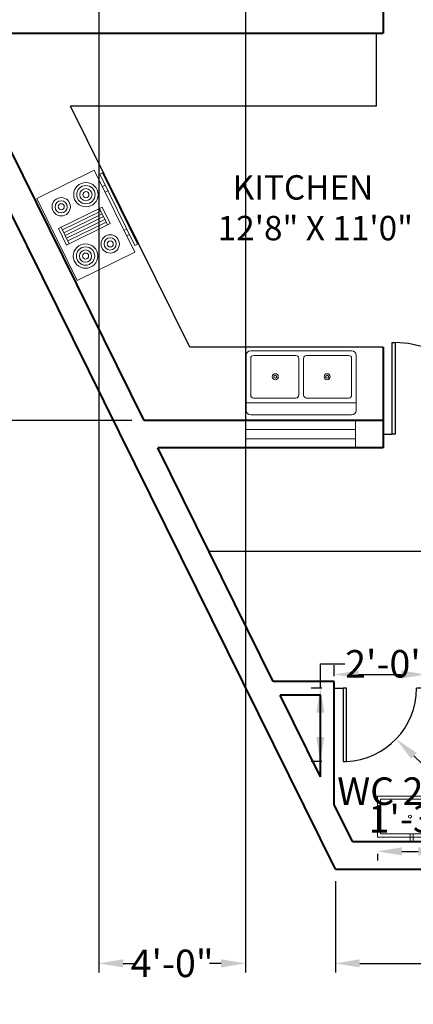
# Model space of a CAD drawing. Units: inches. Extents: x 927 to 1540, y 259 to 890.
# Tile 2 of 4: x 1137 to 1265, y 259 to 582. Entities that reach past the tile are written whole.
import ezdxf

# ---------------------------------------------------------------- set-up
doc = ezdxf.new("R2010")
doc.units = ezdxf.units.IN
doc.header["$MEASUREMENT"] = 0
for name, color, linetype, lineweight in [('A-ANNO-DIMS', 2, 'Continuous', 18), ('A-AREA-IDEN', 7, 'Continuous', 25), ('A-DOOR', 3, 'Continuous', 25), ('A-EQPM', 8, 'Continuous', 18), ('A-EQPM-PATT', 8, 'Continuous', 13), ('A-FLOR-CASE', 9, 'Continuous', 25), ('A-FLOR-FIXT', 9, 'Continuous', 18), ('A-FLOR-STRS', 7, 'Continuous', 25), ('A-GLAZ', 4, 'Continuous', 18), ('A-WALL', 7, 'Continuous', 40)]:
    doc.layers.add(name, color=color, linetype=linetype, lineweight=lineweight)
doc.styles.get("Standard").update_dxf_attribs({"font": 'arial.ttf'})
doc.dimstyles.get("Standard").update_dxf_attribs({"dimtxt": 9, "dimasz": 8, "dimexe": 3, "dimexo": 4, "dimgap": 0.09, "dimtad": 0, "dimtih": 1, "dimtoh": 1, "dimdec": 0, "dimzin": 0, "dimdsep": 46, "dimlunit": 3, "dimtxsty": 'Standard', "dimcen": 0.09, "dimadec": 0, "dimazin": 0, "dimtfac": 1, "dimtdec": 0, "dimtofl": 0, "dimtmove": 0, "dimatfit": 3, "dimfxl": 1, "dimtolj": 1, "dimtzin": 0, "dimarcsym": 0})

# ---------------------------------------------------------------- blocks, each defined once
blk = doc.blocks.new('DOOR-SINGLE-36-OPENING')
for p, q in [((3, 0), (3, 30)), ((3, 30), (4, 30)), ((4, 30), (4, 0)), ((0, 0), (3, 0)), ((4, 0), (3, 0)), ((36, 0), (33, 0))]:
    blk.add_line(p, q)
blk.add_arc((4, 0.98), 29.02, 358.058, 90)
blk = doc.blocks.new('DOOR-SINGLE-30-OPENING')
for p, q in [((0, 24), (3, 24)), ((3, 24), (3, 0)), ((4, 24), (3, 24)), ((4, 0), (4, 24)), ((30, 24), (27, 24)), ((3, 0), (4, 0))]:
    blk.add_line(p, q)
blk.add_arc((2.98, 24), 24.02, 272.4378, 0)
blk = doc.blocks.new('LAVATORY-RECTANGULAR')
for p, q in [((10.69, 2.5), (10.69, 0)), ((11.69, 2.5), (11.69, 0))]:
    blk.add_line(p, q)
for points in [[(0, 1.5), (21.39, 1.5), (21.39, 14.9), (0, 14.9)], [(1, 2.5), (20.39, 2.5), (20.39, 13.9), (1, 13.9)]]:
    blk.add_lwpolyline(points, close=True)
blk.add_circle((10.69, 8.2), 0.491)
blk = doc.blocks.new('WINDOW-36')
for p, q in [((0, 9), (0, 0)), ((36, 9), (36, 0)), ((0, 6), (36, 6)), ((0, 3), (36, 3))]:
    blk.add_line(p, q)
blk = doc.blocks.new('*D34')
at = {"layer": 'A-ANNO-DIMS', "color": 0, "lineweight": -2, "transparency": 16777216}
for p, q in [((1239.48, 366.64), (1239.48, 370.14)), ((1269.48, 366.64), (1269.48, 370.14)), ((1247.48, 367.14), (1261.48, 367.14)), ((1269.48, 367.14), (1277.48, 367.14))]:
    blk.add_line(p, q, dxfattribs=at)
at = {"layer": 'A-ANNO-DIMS', "color": 0, "lineweight": 100, "transparency": 16777216}
for points in [[(1247.48, 368.47), (1247.48, 365.81), (1239.48, 367.14)], [(1261.48, 368.47), (1261.48, 365.81), (1269.48, 367.14)]]:
    blk.add_solid(points, dxfattribs=at)
at = {"layer": 'Defpoints', "color": 0, "lineweight": 100, "transparency": 16777216}
for p in [(1269.48, 367.14), (1239.48, 362.64), (1269.48, 362.64)]:
    blk.add_point(p, dxfattribs=at)
at = {"layer": 'A-ANNO-DIMS', "color": 0, "transparency": 16777216, "insert": (1349.47, 367.14), "char_height": 9, "attachment_point": 5}
blk.add_mtext('\\A1;TOILET DOOR 2\'-6" TYP.', dxfattribs=at)
blk = doc.blocks.new('*D35')
at = {"layer": 'A-ANNO-DIMS', "color": 0, "lineweight": -2, "transparency": 16777216}
for p, q in [((1234.98, 362.64), (1234.98, 370.64)), ((1234.98, 370.64), (1242.98, 370.64)), ((1235.48, 362.64), (1231.98, 362.64)), ((1234.98, 346.64), (1234.98, 354.64)), ((1235.48, 338.64), (1231.98, 338.64))]:
    blk.add_line(p, q, dxfattribs=at)
at = {"layer": 'A-ANNO-DIMS', "color": 0, "lineweight": 100, "transparency": 16777216}
for points in [[(1233.64, 354.64), (1236.31, 354.64), (1234.98, 362.64)], [(1233.64, 346.64), (1236.31, 346.64), (1234.98, 338.64)]]:
    blk.add_solid(points, dxfattribs=at)
at = {"layer": 'Defpoints', "color": 0, "lineweight": 100, "transparency": 16777216}
for p in [(1234.98, 362.64), (1239.48, 362.64), (1239.48, 338.64)]:
    blk.add_point(p, dxfattribs=at)
at = {"layer": 'A-ANNO-DIMS', "color": 0, "transparency": 16777216, "insert": (1270.57, 370.64), "char_height": 9, "attachment_point": 5}
blk.add_mtext('\\A1;2\'-0" TYP.', dxfattribs=at)
blk = doc.blocks.new('*D44')
at = {"layer": 'A-ANNO-DIMS', "color": 0, "lineweight": -2, "transparency": 16777216}
for p, q in [((1279.6, 345.44), (1275.65, 345.44)), ((1278.65, 337.44), (1278.65, 333.66)), ((1278.65, 320.39), (1278.65, 324.17)), ((1279.6, 312.39), (1275.65, 312.39))]:
    blk.add_line(p, q, dxfattribs=at)
at = {"layer": 'A-ANNO-DIMS', "color": 0, "lineweight": 100, "transparency": 16777216}
for points in [[(1277.31, 337.44), (1279.98, 337.44), (1278.65, 345.44)], [(1277.31, 320.39), (1279.98, 320.39), (1278.65, 312.39)]]:
    blk.add_solid(points, dxfattribs=at)
at = {"layer": 'Defpoints', "color": 0, "lineweight": 100, "transparency": 16777216}
for p in [(1283.6, 345.44), (1278.65, 312.39), (1283.6, 312.39)]:
    blk.add_point(p, dxfattribs=at)
at = {"layer": 'A-ANNO-DIMS', "color": 0, "transparency": 16777216, "insert": (1278.65, 328.91), "char_height": 9, "attachment_point": 5}
blk.add_mtext('\\A1;WC 2\'-9" TYP.', dxfattribs=at)
blk = doc.blocks.new('*D46')
at = {"layer": 'A-ANNO-DIMS', "color": 0, "lineweight": -2, "transparency": 16777216}
for p, q in [((1253.64, 308.39), (1253.64, 306.18)), ((1261.64, 309.18), (1267.03, 309.18)), ((1275.03, 309.18), (1283.03, 309.18)), ((1275.03, 308.39), (1275.03, 306.18))]:
    blk.add_line(p, q, dxfattribs=at)
at = {"layer": 'A-ANNO-DIMS', "color": 0, "lineweight": 100, "transparency": 16777216}
for points in [[(1261.64, 310.52), (1261.64, 307.85), (1253.64, 309.18)], [(1267.03, 310.52), (1267.03, 307.85), (1275.03, 309.18)]]:
    blk.add_solid(points, dxfattribs=at)
at = {"layer": 'Defpoints', "color": 0, "lineweight": 100, "transparency": 16777216}
for p in [(1253.64, 312.39), (1275.03, 312.39), (1275.03, 309.18)]:
    blk.add_point(p, dxfattribs=at)
at = {"layer": 'A-ANNO-DIMS', "color": 0, "transparency": 16777216, "insert": (1341.45, 309.18), "char_height": 9, "attachment_point": 5}
blk.add_mtext('\\A1;BASIN 1\'-9 1/2" TYP.', dxfattribs=at)
blk = doc.blocks.new('*D47')
at = {"layer": 'A-ANNO-DIMS', "color": 0, "lineweight": -2, "transparency": 16777216}
for p, q in [((1278.23, 335.29), (1278.23, 343.29)), ((1279.03, 327.29), (1281.23, 327.29)), ((1279.03, 312.39), (1281.23, 312.39)), ((1278.23, 304.39), (1278.23, 296.39))]:
    blk.add_line(p, q, dxfattribs=at)
at = {"layer": 'A-ANNO-DIMS', "color": 0, "lineweight": 100, "transparency": 16777216}
for points in [[(1276.9, 335.29), (1279.57, 335.29), (1278.23, 327.29)], [(1276.9, 304.39), (1279.57, 304.39), (1278.23, 312.39)]]:
    blk.add_solid(points, dxfattribs=at)
at = {"layer": 'Defpoints', "color": 0, "lineweight": 100, "transparency": 16777216}
for p in [(1275.03, 327.29), (1278.23, 327.29), (1275.03, 312.39)]:
    blk.add_point(p, dxfattribs=at)
at = {"layer": 'A-ANNO-DIMS', "color": 0, "transparency": 16777216, "insert": (1278.23, 319.84), "char_height": 9, "attachment_point": 5}
blk.add_mtext('\\A1;1\'-3" TYP.', dxfattribs=at)
blk = doc.blocks.new('*D52')
at = {"layer": 'A-ANNO-DIMS', "color": 0, "lineweight": -2, "transparency": 16777216}
for p, q in [((1239.89, 299.39), (1239.89, 269.49)), ((1414.48, 299.39), (1414.48, 269.49)), ((1247.89, 272.49), (1301.57, 272.49)), ((1406.48, 272.49), (1352.79, 272.49))]:
    blk.add_line(p, q, dxfattribs=at)
at = {"layer": 'A-ANNO-DIMS', "color": 0, "lineweight": 100, "transparency": 16777216}
for points in [[(1247.89, 273.82), (1247.89, 271.16), (1239.89, 272.49)], [(1406.48, 273.82), (1406.48, 271.16), (1414.48, 272.49)]]:
    blk.add_solid(points, dxfattribs=at)
at = {"layer": 'Defpoints', "color": 0, "lineweight": 100, "transparency": 16777216}
for p in [(1239.89, 303.39), (1414.48, 303.39), (1414.48, 272.49)]:
    blk.add_point(p, dxfattribs=at)
at = {"layer": 'A-ANNO-DIMS', "color": 0, "transparency": 16777216, "insert": (1327.18, 272.49), "char_height": 9, "attachment_point": 5}
blk.add_mtext('\\A1;14\'-6 1/2"', dxfattribs=at)
blk = doc.blocks.new('*D57')
at = {"layer": 'A-ANNO-DIMS', "color": 0, "lineweight": -2, "transparency": 16777216}
for p, q in [((1110.59, 577.32), (951.4, 577.32)), ((954.4, 569.32), (954.4, 518.54)), ((954.4, 458.39), (954.4, 509.17)), ((1173.3, 450.39), (951.4, 450.39))]:
    blk.add_line(p, q, dxfattribs=at)
at = {"layer": 'A-ANNO-DIMS', "color": 0, "lineweight": 100, "transparency": 16777216}
for points in [[(953.07, 569.32), (955.74, 569.32), (954.4, 577.32)], [(953.07, 458.39), (955.74, 458.39), (954.4, 450.39)]]:
    blk.add_solid(points, dxfattribs=at)
at = {"layer": 'Defpoints', "color": 0, "lineweight": 100, "transparency": 16777216}
for p in [(1114.59, 577.32), (954.4, 450.39), (1177.3, 450.39)]:
    blk.add_point(p, dxfattribs=at)
at = {"layer": 'A-ANNO-DIMS', "color": 0, "transparency": 16777216, "insert": (954.4, 513.86), "char_height": 9, "attachment_point": 5}
blk.add_mtext('\\A1;10\'-7"', dxfattribs=at)
blk = doc.blocks.new('*D58')
at = {"layer": 'A-ANNO-DIMS', "color": 0, "lineweight": -2, "transparency": 16777216}
for p, q in [((1162.48, 728.87), (1162.48, 269.49)), ((1210.48, 728.87), (1210.48, 269.49)), ((1170.48, 272.49), (1174.24, 272.49)), ((1202.48, 272.49), (1198.71, 272.49))]:
    blk.add_line(p, q, dxfattribs=at)
at = {"layer": 'A-ANNO-DIMS', "color": 0, "lineweight": 100, "transparency": 16777216}
for points in [[(1170.48, 273.82), (1170.48, 271.16), (1162.48, 272.49)], [(1202.48, 273.82), (1202.48, 271.16), (1210.48, 272.49)]]:
    blk.add_solid(points, dxfattribs=at)
at = {"layer": 'Defpoints', "color": 0, "lineweight": 100, "transparency": 16777216}
for p in [(1162.48, 732.87), (1210.48, 732.87), (1210.48, 272.49)]:
    blk.add_point(p, dxfattribs=at)
at = {"layer": 'A-ANNO-DIMS', "color": 0, "transparency": 16777216, "insert": (1186.48, 272.49), "char_height": 9, "attachment_point": 5}
blk.add_mtext('\\A1;4\'-0"', dxfattribs=at)
blk = doc.blocks.new('*D60')
at = {"layer": 'A-ANNO-DIMS', "color": 0, "lineweight": -2, "transparency": 16777216}
for p, q in [((1242.37, 362.64), (1242.55, 362.64)), ((1242.46, 362.55), (1242.46, 362.73)), ((1271.35, 334.95), (1265.58, 340.49)), ((1279.35, 334.95), (1271.35, 334.95))]:
    blk.add_line(p, q, dxfattribs=at)
at = {"layer": 'A-ANNO-DIMS', "color": 0, "lineweight": 100, "transparency": 16777216}
blk.add_solid([(1266.5, 341.45), (1264.65, 339.52), (1259.8, 346.02)], dxfattribs=at)
at = {"layer": 'Defpoints', "color": 0, "lineweight": 100, "transparency": 16777216}
for p in [(1242.46, 362.64), (1259.8, 346.02)]:
    blk.add_point(p, dxfattribs=at)
at = {"layer": 'A-ANNO-DIMS', "color": 0, "transparency": 16777216, "insert": (1295.71, 334.95), "char_height": 9, "attachment_point": 5}
blk.add_mtext('\\A1;R2\'-0"', dxfattribs=at)

msp = doc.modelspace()

# ---------------------------------------------------------------- hatches: boundary and pattern name
at = {"layer": 'A-EQPM-PATT'}
h = msp.add_hatch(dxfattribs=at)
h.set_pattern_fill('ANSI31', color=256, scale=8.044591, angle=-18.78217, style=0)
h.paths.add_polyline_path([(1152.78, 508.3), (1165.34, 514.48), (1162.69, 519.86), (1150.13, 513.68)])

# ---------------------------------------------------------------- linework, layer by layer
at = {"layer": 'A-EQPM'}
for p, q in [((1142.14, 523.12), (1160.98, 532.4)), ((1160.98, 532.4), (1174.23, 505.48)), ((1162.76, 531.04), (1163.66, 531.49)), ((1174.25, 507.72), (1162.76, 531.04)), ((1163.66, 531.49), (1175.14, 508.16)), ((1163.63, 527.01), (1164.53, 527.46)), ((1155.39, 496.21), (1142.14, 523.12)), ((1165.41, 525.66), (1164.51, 525.22)), ((1149.24, 513.24), (1163.59, 520.31)), ((1162.69, 519.86), (1165.34, 514.48)), ((1163.59, 520.31), (1166.24, 514.92)), ((1151.89, 507.86), (1149.24, 513.24)), ((1152.78, 508.3), (1150.13, 513.68)), ((1166.24, 514.92), (1151.89, 507.86)), ((1171.6, 513.1), (1170.7, 512.66)), ((1171.58, 510.87), (1172.48, 511.31)), ((1175.14, 508.16), (1174.25, 507.72)), ((1174.23, 505.48), (1155.39, 496.21))]:
    msp.add_line(p, q, dxfattribs=at)
for centre, radius in [((1158.25, 524.36), 4), ((1158.25, 524.36), 3), ((1158.25, 524.36), 2), ((1150.17, 520.39), 3), ((1158.25, 524.36), 1), ((1150.17, 520.39), 2), ((1150.17, 520.39), 1), ((1166.2, 508.22), 3), ((1166.2, 508.22), 2), ((1158.13, 504.24), 4), ((1158.13, 504.24), 3), ((1166.2, 508.22), 1), ((1158.13, 504.24), 2), ((1158.13, 504.24), 1)]:
    msp.add_circle(centre, radius, dxfattribs=at)
at = {"layer": 'A-FLOR-CASE'}
for p, q in [((1253.23, 577.32), (1253.23, 553.32)), ((1253.23, 553.32), (1153.22, 553.32)), ((1192.21, 474.39), (1153.22, 553.32)), ((1255.48, 474.39), (1192.21, 474.39))]:
    msp.add_line(p, q, dxfattribs=at)
at = {"layer": 'A-FLOR-FIXT'}
for p, q in [((1227.95, 458.68), (1227.95, 470.68)), ((1229.45, 470.68), (1229.45, 458.68)), ((1246.7, 456.18), (1210.7, 456.18))]:
    msp.add_line(p, q, dxfattribs=at)
for points in [[(1210.7, 453.68), (1210.7, 471.68)], [(1212.2, 473.18), (1245.2, 473.18)], [(1213.2, 471.68), (1226.95, 471.68)], [(1230.45, 471.68), (1244.2, 471.68)], [(1246.7, 471.68), (1246.7, 453.68)], [(1212.2, 458.68), (1212.2, 470.68)], [(1245.2, 470.68), (1245.2, 458.68)], [(1226.95, 457.68), (1213.2, 457.68)], [(1244.2, 457.68), (1230.45, 457.68)], [(1245.2, 452.18), (1212.2, 452.18)]]:
    msp.add_lwpolyline(points, dxfattribs=at)
for centre, radius in [((1220.2, 464.68), 1), ((1220.2, 464.68), 0.5), ((1237.2, 464.68), 1), ((1237.2, 464.68), 0.5)]:
    msp.add_circle(centre, radius, dxfattribs=at)
for centre, radius, start, end in [((1212.2, 471.68), 1.5, 90, 180), ((1213.2, 470.68), 1, 90, 180), ((1226.95, 470.68), 1, 0, 90), ((1230.45, 470.68), 1, 90, 180), ((1244.2, 470.68), 1, 0, 90), ((1245.2, 471.68), 1.5, 0, 90), ((1213.2, 458.68), 1, 180, 270), ((1226.95, 458.68), 1, 270, 0), ((1230.45, 458.68), 1, 180, 270), ((1244.2, 458.68), 1, 270, 0), ((1212.2, 453.68), 1.5, 180, 270), ((1245.2, 453.68), 1.5, 270, 0)]:
    msp.add_arc(centre, radius, start, end, dxfattribs=at)
at = {"layer": 'A-FLOR-STRS'}
msp.add_line((1371.48, 407.39), (1198.54, 407.39), dxfattribs=at)
at = {"layer": 'A-WALL'}
for p, q in [((1239.89, 303.39), (985.3, 818.67)), ((1255.48, 586.06), (1255.48, 577.32)), ((1114.59, 577.32), (1255.48, 577.32)), ((1177.3, 450.39), (1114.59, 577.32)), ((1255.48, 474.39), (1255.48, 441.39)), ((1255.48, 450.39), (1177.3, 450.39)), ((1255.48, 441.39), (1181.75, 441.39)), ((1219.54, 364.89), (1181.75, 441.39)), ((1239.48, 364.89), (1219.54, 364.89)), ((1239.48, 360.39), (1239.48, 364.89)), ((1234.98, 360.39), (1221.77, 360.39)), ((1234.98, 333.65), (1221.77, 360.39)), ((1234.98, 333.65), (1234.98, 360.39)), ((1239.48, 324.54), (1239.48, 360.39)), ((1245.48, 312.39), (1239.48, 324.54)), ((1245.48, 312.39), (1311.48, 312.39)), ((1239.89, 303.39), (1324.48, 303.39))]:
    msp.add_line(p, q, dxfattribs=at)

# ---------------------------------------------------------------- block references
at = {"layer": 'A-DOOR'}
for name, p in [('DOOR-SINGLE-36-OPENING', (1255.48, 445.89)), ('DOOR-SINGLE-30-OPENING', (1239.48, 338.64))]:
    msp.add_blockref(name, p, dxfattribs=at)
at = {"layer": 'A-FLOR-FIXT'}
msp.add_blockref('LAVATORY-RECTANGULAR', (1253.64, 312.39), dxfattribs=at)
at = {"layer": 'A-GLAZ', "extrusion": (0, 0, -1), "zscale": -1}
msp.add_blockref('WINDOW-36', (-1246.48, 441.39), dxfattribs=at)

# ---------------------------------------------------------------- texts
at = {"layer": 'A-AREA-IDEN', "insert": (1201.38, 530.74), "char_height": 8, "attachment_point": 1}
msp.add_mtext_dynamic_manual_height_columns('  KITCHEN\\P12\'8" X 11\'0"', width=78.5806, gutter_width=1, heights=[0], dxfattribs=at)

# ---------------------------------------------------------------- dimensions: what is measured, and where the dimension line sits
at = {"layer": 'A-ANNO-DIMS'}
for base, p1, p2, picture, middle in [((1210.48, 272.49), (1162.48, 732.87), (1210.48, 732.87), '*D58', (1186.48, 272.49)), ((1414.48, 272.49), (1239.89, 303.39), (1414.48, 303.39), '*D52', (1327.18, 272.49))]:
    dim = msp.add_linear_dim(base=base, p1=p1, p2=p2, dimstyle='Standard', override={"dimdec": 1, "dimlfac": 1, "dimrnd": 0, "dimzin": 1, "dimdsep": 46, "dimlunit": 4, "dimfrac": 2}, dxfattribs=at)
    dim.commit()
    dim.dimension.update_dxf_attribs({"geometry": picture, "text_midpoint": middle})
dim = msp.add_linear_dim(base=(954.4, 450.39), p1=(1114.59, 577.32), p2=(1177.3, 450.39), angle=90, dimstyle='Standard', override={"dimdec": 1, "dimlfac": 1, "dimrnd": 0, "dimzin": 1, "dimdsep": 46, "dimlunit": 4, "dimfrac": 2}, dxfattribs=at)
dim.commit()
dim.dimension.update_dxf_attribs({"geometry": '*D57', "text_midpoint": (954.4, 513.86)})
for base, p1, p2, text, picture, middle in [((1269.48, 367.14), (1239.48, 362.64), (1269.48, 362.64), 'TOILET DOOR <> TYP.', '*D34', (1349.47, 367.14)), ((1275.03, 309.18), (1253.64, 312.39), (1275.03, 312.39), 'BASIN <> TYP.', '*D46', (1341.45, 309.18))]:
    dim = msp.add_linear_dim(base=base, p1=p1, p2=p2, text=text, dimstyle='Standard', override={"dimdec": 1, "dimlfac": 1, "dimrnd": 0, "dimzin": 1, "dimdsep": 46, "dimlunit": 4, "dimfrac": 2}, dxfattribs=at)
    dim.commit()
    dim.dimension.update_dxf_attribs({"geometry": picture, "text_midpoint": middle})
for base, p1, p2, angle, text, picture, middle in [((1234.98, 362.64), (1239.48, 338.64), (1239.48, 362.64), 90, '<> TYP.', '*D35', (1270.57, 370.64)), ((1278.6468, 312.3913), (1283.6038, 345.4376), (1283.6038, 312.3913), 270, 'WC <> TYP.', '*D44', (1278.6468, 328.9144)), ((1278.23, 327.29), (1275.03, 312.39), (1275.03, 327.29), 90, '<> TYP.', '*D47', (1278.23, 319.84))]:
    dim = msp.add_linear_dim(base=base, p1=p1, p2=p2, angle=angle, text=text, dimstyle='Standard', override={"dimdec": 1, "dimlfac": 1, "dimrnd": 0, "dimzin": 1, "dimdsep": 46, "dimlunit": 4, "dimfrac": 2}, dxfattribs=at)
    dim.commit()
    dim.dimension.update_dxf_attribs({"geometry": picture, "text_midpoint": middle})
dim = msp.add_radius_dim(center=(1242.46, 362.64), mpoint=(1259.8, 346.02), dimstyle='Standard', override={"dimdec": 1, "dimlfac": 1, "dimrnd": 0, "dimzin": 1, "dimdsep": 46, "dimlunit": 4, "dimfrac": 2}, dxfattribs=at)
dim.commit()
dim.dimension.update_dxf_attribs({"geometry": '*D60', "text_midpoint": (1295.71, 334.95)})

doc.saveas('drawing.dxf')
